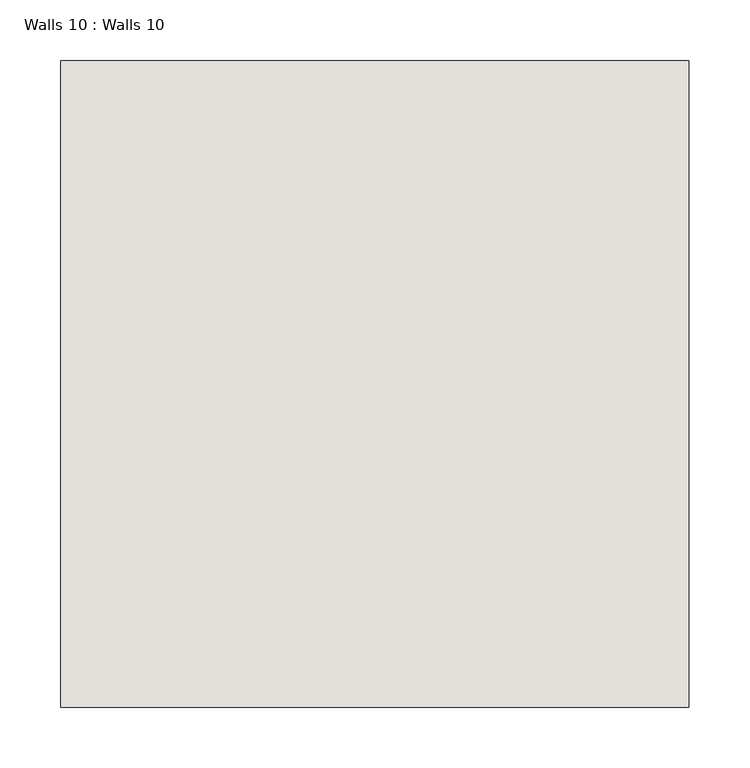
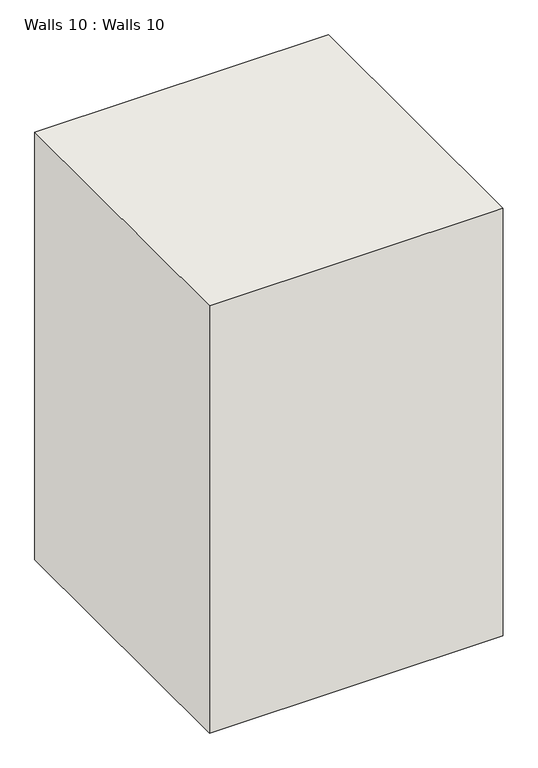
"""IFC4 building model written with IfcOpenShell, lengths in millimetres: wall geometry, Walls 10 : Walls 10."""

from ifc_helpers import new_model, si_unit, origin, origin_with_axes, place, context, project, spatial, polyline, outline, extrude, source, transform, mapped, element, save


def walls_10_walls_10_b49e789a(model_context):
    return source(origin(), model_context, "Body", "SweptSolid", [
        extrude(outline(polyline([(-8668.9478722, -7390.0501996), (-8668.9478722, -7923.4501996), (-9187.2996792, -7923.4501996), (-9187.2996792, -7390.0501996), (-8668.9478722, -7390.0501996)])), origin_with_axes(), (0.0, 0.0, 1.0), 796.9860094),
    ])


if __name__ == "__main__":
    model = new_model("IFC4")
    model_context = context("Model", 3, world=origin())
    ifc_project = project(units=[si_unit("LENGTHUNIT", "METRE", prefix="MILLI")], contexts=[model_context])
    site = spatial("IfcSite", under=ifc_project)
    building = spatial("IfcBuilding", under=site)
    placement = place(None, origin())
    walls_10_walls_10_shape = walls_10_walls_10_b49e789a(model_context)
    element("IfcWall", 1, ObjectType="Walls 10 : Walls 10", at=placement, inside=building, context=model_context, shape_type="MappedRepresentation", body=[
        mapped(walls_10_walls_10_shape, transform((0.0, 0.0, 0.0), x_axis=(1.0, 0.0, 0.0), y_axis=(0.0, 1.0, 0.0), z_axis=(0.0, 0.0, 1.0))),
    ])
    save(model, "model.ifc")

# Revit data of these elements
# Element 1 (IfcWall, "Walls 10 : Walls 10")
#   Materials on its faces: "Default Wall"
# Materials
#   "Default Wall": colour RGB 80 80 80, transparency 0
